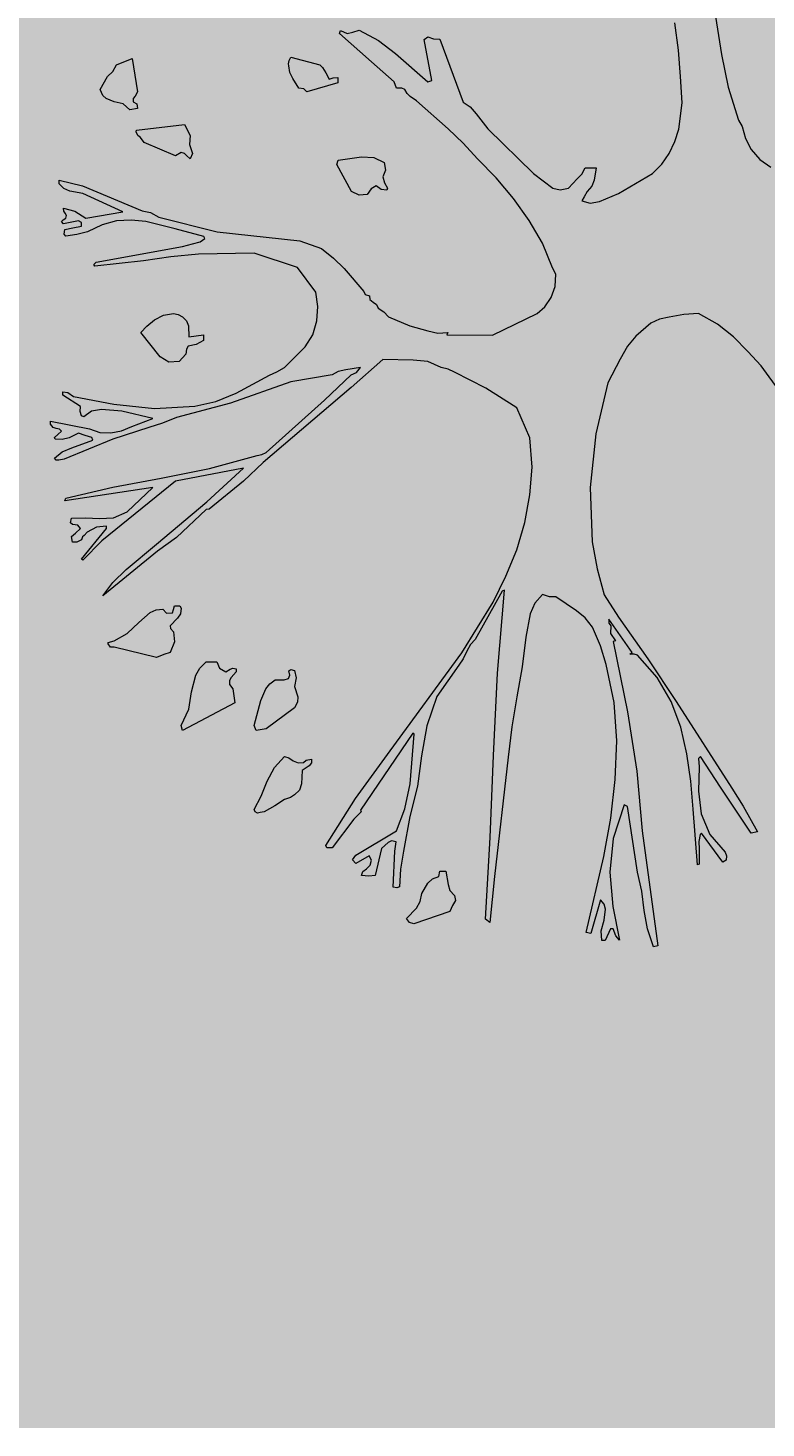
# Model space of a CAD drawing. Units: inches. Extents: x 84 to 1044, y -280 to 906.
# Tile 87 of 105: x 870 to 883, y 400 to 426. Entities that reach past the tile are written whole.
import ezdxf

# ---------------------------------------------------------------- set-up
doc = ezdxf.new("R2010")
doc.units = ezdxf.units.IN
doc.layers.add('A-ANNO-DIMS', color=2, linetype='Continuous', lineweight=18)
doc.layers.add('L-PLNT', color=114, linetype='Continuous', lineweight=15)
doc.layers.add('L-PLNT-PATT', color=9, linetype='Continuous', lineweight=9, true_color=0xafd9aa)
doc.styles.get("Standard").update_dxf_attribs({"font": 'arial.ttf'})
doc.dimstyles.get("Standard").update_dxf_attribs({"dimtxt": 0.18, "dimasz": 0.18, "dimexe": 0.18, "dimexo": 0.0625, "dimgap": 0.09, "dimtad": 0, "dimtih": 1, "dimtoh": 1, "dimdec": 4, "dimzin": 0, "dimdsep": 46, "dimtxsty": 'Standard', "dimcen": 0.09, "dimadec": 0, "dimazin": 0, "dimtfac": 1, "dimtdec": 4, "dimtofl": 0, "dimtmove": 0, "dimatfit": 3, "dimfxl": 1, "dimtolj": 1, "dimtzin": 0, "dimarcsym": 0})

# ---------------------------------------------------------------- blocks, each defined once
blk = doc.blocks.new('A$C37E508DF')
for p, q in [((0.7911, 1.1436), (0.8027, 1.0677)), ((0.3456, 1.093), (0.3469, 1.0964)), ((0.3842, 1.0591), (0.3456, 1.093)), ((0.3469, 1.0964), (0.355, 1.093)), ((0.355, 1.093), (0.3619, 1.0943)), ((0.3619, 1.0943), (0.3692, 1.0968)), ((0.3692, 1.0968), (0.3923, 1.0844)), ((0.7512, 1.0728), (0.7469, 1.1054)), ((0.3923, 1.0844), (0.4129, 1.069)), ((0.4472, 1.0857), (0.4515, 1.0887)), ((0.4562, 1.0364), (0.4472, 1.0857)), ((0.4515, 1.0887), (0.4584, 1.0865)), ((0.4584, 1.0865), (0.4657, 1.0861)), ((0.4657, 1.0861), (0.4939, 1.0107)), ((0.7538, 1.0415), (0.7512, 1.0728)), ((0.0789, 1.0552), (0.0978, 1.063)), ((0.0978, 1.063), (0.1042, 1.0231)), ((0.2847, 1.0565), (0.2856, 1.0604)), ((0.2851, 1.054), (0.2847, 1.0565)), ((0.2856, 1.0604), (0.2877, 1.0647)), ((0.2877, 1.0647), (0.3224, 1.0552)), ((0.4112, 1.0351), (0.3842, 1.0591)), ((0.4129, 1.069), (0.4515, 1.0351)), ((0.8027, 1.0677), (0.8108, 1.0287)), ((0.0596, 1.0257), (0.0682, 1.0415)), ((0.0682, 1.0415), (0.0746, 1.0475)), ((0.0746, 1.0475), (0.0789, 1.0552)), ((0.2864, 1.0463), (0.2851, 1.054)), ((0.2899, 1.039), (0.2864, 1.0463)), ((0.2972, 1.0274), (0.2899, 1.039)), ((0.3224, 1.0552), (0.3255, 1.0522)), ((0.3255, 1.0522), (0.3293, 1.0458)), ((0.3293, 1.0458), (0.3336, 1.0381)), ((0.3336, 1.0381), (0.3383, 1.0398)), ((0.3383, 1.0398), (0.3439, 1.0402)), ((0.3439, 1.0402), (0.3439, 1.0338)), ((0.7559, 1.0098), (0.7538, 1.0415)), ((0.0626, 1.0188), (0.0596, 1.0257)), ((0.1042, 1.0231), (0.1012, 1.018)), ((0.3032, 1.0265), (0.2972, 1.0274)), ((0.3066, 1.0231), (0.3032, 1.0265)), ((0.3439, 1.0338), (0.3066, 1.0231)), ((0.4138, 1.0274), (0.4112, 1.0351)), ((0.4202, 1.0274), (0.4138, 1.0274)), ((0.4241, 1.0257), (0.4202, 1.0274)), ((0.4267, 1.0209), (0.4241, 1.0257)), ((0.4515, 1.0351), (0.4562, 1.0364)), ((0.8108, 1.0287), (0.8233, 0.9892)), ((0.0665, 1.0149), (0.0626, 1.0188)), ((0.0763, 1.0111), (0.0665, 1.0149)), ((0.087, 1.0085), (0.0763, 1.0111)), ((0.0948, 1.0016), (0.087, 1.0085)), ((0.1012, 1.018), (0.099, 1.0149)), ((0.099, 1.0149), (0.099, 1.0111)), ((0.099, 1.0111), (0.1033, 1.0085)), ((0.1033, 1.0085), (0.1042, 1.0029)), ((0.4305, 1.0175), (0.4267, 1.0209)), ((0.4378, 1.0124), (0.4305, 1.0175)), ((0.476, 0.9789), (0.4378, 1.0124)), ((0.4939, 1.0107), (0.5021, 1.0051)), ((0.5021, 1.0051), (0.5094, 0.9969)), ((0.7516, 0.9785), (0.7559, 1.0098)), ((0.1042, 1.0029), (0.0948, 1.0016)), ((0.5094, 0.9969), (0.5231, 0.9789)), ((0.8233, 0.9892), (0.8275, 0.9815)), ((0.1025, 0.9751), (0.1029, 0.9772)), ((0.1046, 0.9708), (0.1025, 0.9751)), ((0.1029, 0.9772), (0.1604, 0.9841)), ((0.1604, 0.9841), (0.1672, 0.9708)), ((0.4939, 0.9618), (0.476, 0.9789)), ((0.5231, 0.9789), (0.578, 0.9253)), ((0.7469, 0.9635), (0.7516, 0.9785)), ((0.8275, 0.9815), (0.8314, 0.9673)), ((0.1076, 0.9682), (0.1046, 0.9708)), ((0.1119, 0.9626), (0.1076, 0.9682)), ((0.1496, 0.9463), (0.1119, 0.9626)), ((0.1672, 0.9708), (0.1664, 0.9601)), ((0.1664, 0.9601), (0.1698, 0.9493)), ((0.5111, 0.9429), (0.4939, 0.9618)), ((0.7401, 0.9493), (0.7469, 0.9635)), ((0.8314, 0.9673), (0.8383, 0.954)), ((0.1565, 0.9506), (0.1496, 0.9463)), ((0.1604, 0.9493), (0.1565, 0.9506)), ((0.1629, 0.9468), (0.1604, 0.9493)), ((0.1672, 0.9429), (0.1629, 0.9468)), ((0.1698, 0.9493), (0.1672, 0.9429)), ((0.3426, 0.936), (0.3443, 0.9412)), ((0.3443, 0.9412), (0.3722, 0.9451)), ((0.3722, 0.9451), (0.3868, 0.9446)), ((0.3868, 0.9446), (0.3992, 0.9386)), ((0.3992, 0.9386), (0.4009, 0.9292)), ((0.5334, 0.9202), (0.5111, 0.9429)), ((0.7315, 0.9365), (0.7401, 0.9493)), ((0.8383, 0.954), (0.8486, 0.942)), ((0.8486, 0.942), (0.8619, 0.933)), ((0.3602, 0.9039), (0.3426, 0.936)), ((0.4009, 0.9292), (0.3975, 0.9215)), ((0.3975, 0.9215), (0.3996, 0.9142)), ((0.578, 0.9253), (0.6011, 0.9077)), ((0.6303, 0.9189), (0.6359, 0.9245)), ((0.6359, 0.9245), (0.6397, 0.9322)), ((0.6397, 0.9322), (0.653, 0.9322)), ((0.653, 0.9322), (0.6505, 0.9172)), ((0.6796, 0.9013), (0.7203, 0.9253)), ((0.7203, 0.9253), (0.7315, 0.9365)), ((0.0103, 0.9129), (0.0103, 0.9172)), ((0.0103, 0.9172), (0.0382, 0.9107)), ((0.0159, 0.9073), (0.0103, 0.9129)), ((0.0232, 0.9043), (0.0159, 0.9073)), ((0.0382, 0.9107), (0.1098, 0.8807)), ((0.3838, 0.9069), (0.379, 0.9)), ((0.3898, 0.9107), (0.3838, 0.9069)), ((0.3958, 0.906), (0.3898, 0.9107)), ((0.4026, 0.9052), (0.3958, 0.906)), ((0.3996, 0.9142), (0.4031, 0.9077)), ((0.4031, 0.9077), (0.4026, 0.9052)), ((0.554, 0.8953), (0.5334, 0.9202)), ((0.6011, 0.9077), (0.6097, 0.9056)), ((0.6097, 0.9056), (0.6196, 0.9077)), ((0.6196, 0.9077), (0.6303, 0.9189)), ((0.6479, 0.9103), (0.6423, 0.9039)), ((0.6505, 0.9172), (0.6479, 0.9103)), ((0.0386, 0.9013), (0.0232, 0.9043)), ((0.0866, 0.8794), (0.0386, 0.9013)), ((0.3692, 0.8992), (0.3602, 0.9039)), ((0.379, 0.9), (0.3692, 0.8992)), ((0.5728, 0.8691), (0.554, 0.8953)), ((0.6384, 0.8974), (0.6359, 0.8927)), ((0.6359, 0.8927), (0.6457, 0.8897)), ((0.6423, 0.9039), (0.6384, 0.8974)), ((0.6457, 0.8897), (0.6569, 0.8919)), ((0.6569, 0.8919), (0.6796, 0.9013)), ((0.015, 0.87), (0.0184, 0.8717)), ((0.0159, 0.8803), (0.0154, 0.8837)), ((0.0154, 0.8837), (0.0292, 0.8803)), ((0.0176, 0.8777), (0.0159, 0.8803)), ((0.0193, 0.8752), (0.0176, 0.8777)), ((0.0184, 0.8717), (0.0193, 0.8752)), ((0.0292, 0.8803), (0.0424, 0.8717)), ((0.0424, 0.8717), (0.0866, 0.8794)), ((0.1098, 0.8807), (0.1196, 0.8786)), ((0.1196, 0.8786), (0.1295, 0.873)), ((0.1295, 0.873), (0.1994, 0.8554)), ((0.0133, 0.8679), (0.015, 0.87)), ((0.0154, 0.8649), (0.0133, 0.8679)), ((0.0334, 0.8687), (0.0154, 0.8649)), ((0.0163, 0.8529), (0.0171, 0.8584)), ((0.0171, 0.8584), (0.0266, 0.8602)), ((0.0266, 0.8602), (0.0369, 0.8623)), ((0.0442, 0.8554), (0.0317, 0.8524)), ((0.0369, 0.8666), (0.0334, 0.8687)), ((0.0369, 0.8623), (0.0369, 0.8666)), ((0.0617, 0.864), (0.0442, 0.8554)), ((0.0789, 0.8687), (0.0617, 0.864)), ((0.0965, 0.8696), (0.0789, 0.8687)), ((0.1141, 0.8679), (0.0965, 0.8696)), ((0.1492, 0.8593), (0.1141, 0.8679)), ((0.1835, 0.8499), (0.1492, 0.8593)), ((0.1994, 0.8554), (0.2984, 0.8447)), ((0.5887, 0.8421), (0.5728, 0.8691)), ((0.0184, 0.8503), (0.0163, 0.8529)), ((0.0317, 0.8524), (0.0184, 0.8503)), ((0.0545, 0.8194), (0.1578, 0.8378)), ((0.1578, 0.8378), (0.1698, 0.8413)), ((0.1698, 0.8413), (0.1792, 0.8434)), ((0.1792, 0.8434), (0.1848, 0.8477)), ((0.1848, 0.8477), (0.1835, 0.8499)), ((0.2984, 0.8447), (0.3242, 0.8357)), ((0.6007, 0.8125), (0.5887, 0.8421)), ((0.1441, 0.8258), (0.1111, 0.8207)), ((0.1771, 0.8288), (0.1441, 0.8258)), ((0.2436, 0.8301), (0.1771, 0.8288)), ((0.2954, 0.813), (0.2436, 0.8301)), ((0.3242, 0.8357), (0.3387, 0.8241)), ((0.3387, 0.8241), (0.3512, 0.8117)), ((0.0519, 0.8164), (0.0545, 0.8194)), ((0.0532, 0.8143), (0.0519, 0.8164)), ((0.1111, 0.8207), (0.0532, 0.8143)), ((0.3173, 0.7834), (0.2954, 0.813)), ((0.3512, 0.8117), (0.3748, 0.7842)), ((0.6046, 0.8048), (0.6007, 0.8125)), ((0.6037, 0.7903), (0.6046, 0.8048)), ((0.599, 0.777), (0.6037, 0.7903)), ((0.3199, 0.7662), (0.3173, 0.7834)), ((0.3748, 0.7842), (0.3765, 0.7804)), ((0.3765, 0.7804), (0.3816, 0.7791)), ((0.3816, 0.7791), (0.382, 0.7744)), ((0.382, 0.7744), (0.3859, 0.7714)), ((0.3859, 0.7714), (0.3902, 0.7684)), ((0.5913, 0.7658), (0.599, 0.777)), ((0.1244, 0.7504), (0.1351, 0.7559)), ((0.1351, 0.7559), (0.1471, 0.7577)), ((0.1471, 0.7577), (0.1527, 0.7568)), ((0.1527, 0.7568), (0.1578, 0.7538)), ((0.1578, 0.7538), (0.1629, 0.7491)), ((0.3186, 0.7491), (0.3199, 0.7662)), ((0.3902, 0.7684), (0.3919, 0.7641)), ((0.3919, 0.7641), (0.3988, 0.7598)), ((0.3988, 0.7598), (0.4043, 0.7538)), ((0.4043, 0.7538), (0.4301, 0.7431)), ((0.5287, 0.7319), (0.5823, 0.7577)), ((0.5823, 0.7577), (0.5913, 0.7658)), ((0.7577, 0.7568), (0.7401, 0.7534)), ((0.7752, 0.7577), (0.7577, 0.7568)), ((0.798, 0.7452), (0.7752, 0.7577)), ((0.1081, 0.7349), (0.1153, 0.7427)), ((0.1153, 0.7427), (0.1244, 0.7504)), ((0.1629, 0.7491), (0.1651, 0.7431)), ((0.1651, 0.7431), (0.1655, 0.7298)), ((0.3139, 0.7324), (0.3186, 0.7491)), ((0.4301, 0.7431), (0.4515, 0.7371)), ((0.4515, 0.7371), (0.4635, 0.7341)), ((0.7182, 0.7461), (0.7002, 0.7307)), ((0.7285, 0.7512), (0.7182, 0.7461)), ((0.7401, 0.7534), (0.7285, 0.7512)), ((0.8173, 0.7298), (0.798, 0.7452)), ((0.1312, 0.7058), (0.1081, 0.7349)), ((0.1741, 0.7208), (0.1646, 0.7186)), ((0.1655, 0.7298), (0.1831, 0.7324)), ((0.1831, 0.7255), (0.1741, 0.7208)), ((0.1831, 0.7324), (0.1831, 0.7255)), ((0.3049, 0.7178), (0.3139, 0.7324)), ((0.4635, 0.7341), (0.4755, 0.7349)), ((0.4755, 0.7349), (0.4742, 0.7324)), ((0.4742, 0.7324), (0.5287, 0.7319)), ((0.7002, 0.7307), (0.6903, 0.7186)), ((0.8344, 0.7122), (0.8173, 0.7298)), ((0.1415, 0.6994), (0.1312, 0.7058)), ((0.1621, 0.7092), (0.1539, 0.7002)), ((0.1629, 0.7152), (0.1621, 0.7092)), ((0.1646, 0.7186), (0.1629, 0.7152)), ((0.28, 0.6933), (0.3049, 0.7178)), ((0.6903, 0.7186), (0.6818, 0.7032)), ((0.8503, 0.6951), (0.8344, 0.7122)), ((0.1539, 0.7002), (0.1415, 0.6994)), ((0.262, 0.6839), (0.271, 0.6882)), ((0.271, 0.6882), (0.28, 0.6933)), ((0.3443, 0.6886), (0.337, 0.6843)), ((0.3533, 0.6903), (0.3443, 0.6886)), ((0.3709, 0.6933), (0.3533, 0.6903)), ((0.3975, 0.7028), (0.3598, 0.6693)), ((0.3598, 0.6843), (0.3662, 0.6873)), ((0.3662, 0.6873), (0.3709, 0.6933)), ((0.4339, 0.7019), (0.3975, 0.7028)), ((0.4515, 0.7002), (0.4339, 0.7019)), ((0.4674, 0.6933), (0.4515, 0.7002)), ((0.476, 0.6912), (0.4674, 0.6933)), ((0.4832, 0.6878), (0.476, 0.6912)), ((0.521, 0.6685), (0.4832, 0.6878)), ((0.6818, 0.7032), (0.6667, 0.6749)), ((0.8739, 0.6629), (0.8503, 0.6951)), ((0.2877, 0.6762), (0.2152, 0.6505)), ((0.2221, 0.6625), (0.262, 0.6839)), ((0.337, 0.6843), (0.2877, 0.6762)), ((0.328, 0.6543), (0.3598, 0.6843)), ((0.6667, 0.6749), (0.6526, 0.614)), ((0.0146, 0.6599), (0.0146, 0.6642)), ((0.0146, 0.6642), (0.0206, 0.6633)), ((0.036, 0.6466), (0.0146, 0.6599)), ((0.0206, 0.6633), (0.0274, 0.6586)), ((0.0274, 0.6586), (0.0759, 0.6492)), ((0.1977, 0.6526), (0.2221, 0.6625)), ((0.3598, 0.6693), (0.2543, 0.5797)), ((0.2581, 0.5913), (0.328, 0.6543)), ((0.5578, 0.6449), (0.521, 0.6685)), ((0.0356, 0.6406), (0.036, 0.6466)), ((0.0369, 0.6355), (0.0356, 0.6406)), ((0.0489, 0.641), (0.0399, 0.6342)), ((0.0609, 0.6428), (0.0489, 0.641)), ((0.0853, 0.641), (0.0609, 0.6428)), ((0.0759, 0.6492), (0.1244, 0.644)), ((0.1226, 0.632), (0.0853, 0.641)), ((0.1244, 0.644), (0.1728, 0.647)), ((0.2152, 0.6505), (0.1509, 0.6333)), ((0.1728, 0.647), (0.1977, 0.6526)), ((0.5737, 0.6089), (0.5578, 0.6449)), ((0, 0.629), (0.0467, 0.62)), ((0, 0.6252), (0, 0.629)), ((0.003, 0.6213), (0, 0.6252)), ((0.0069, 0.6204), (0.003, 0.6213)), ((0.0107, 0.6196), (0.0069, 0.6204)), ((0.0399, 0.6342), (0.0369, 0.6355)), ((0.0467, 0.62), (0.0592, 0.6153)), ((0.1175, 0.6213), (0.0746, 0.6076)), ((0.0849, 0.6175), (0.0973, 0.6226)), ((0.0973, 0.6226), (0.1226, 0.632)), ((0.1342, 0.6265), (0.1175, 0.6213)), ((0.1509, 0.6333), (0.1342, 0.6265)), ((0.0047, 0.6093), (0.0086, 0.6132)), ((0.0056, 0.6076), (0.0047, 0.6093)), ((0.0141, 0.6072), (0.0056, 0.6076)), ((0.0086, 0.6132), (0.0133, 0.617)), ((0.0133, 0.617), (0.0107, 0.6196)), ((0.0223, 0.6089), (0.0141, 0.6072)), ((0.0746, 0.6076), (0.0163, 0.5836)), ((0.0334, 0.6145), (0.0223, 0.6089)), ((0.0257, 0.5969), (0.0506, 0.6063)), ((0.0416, 0.6119), (0.0334, 0.6145)), ((0.0493, 0.6093), (0.0416, 0.6119)), ((0.0506, 0.6063), (0.0493, 0.6093)), ((0.0592, 0.6153), (0.072, 0.6149)), ((0.072, 0.6149), (0.0849, 0.6175)), ((0.5763, 0.5741), (0.5737, 0.6089)), ((0.6526, 0.614), (0.6457, 0.5497)), ((0.0047, 0.5849), (0.0141, 0.5921)), ((0.0141, 0.5921), (0.0257, 0.5969)), ((0.1904, 0.5724), (0.2474, 0.5879)), ((0.2474, 0.5879), (0.253, 0.5892)), ((0.253, 0.5892), (0.2581, 0.5913)), ((0.0069, 0.5823), (0.0047, 0.5849)), ((0.0099, 0.5823), (0.0069, 0.5823)), ((0.0163, 0.5836), (0.0099, 0.5823)), ((0.1325, 0.5608), (0.1904, 0.5724)), ((0.2311, 0.5729), (0.1496, 0.557)), ((0.1869, 0.5325), (0.2311, 0.5729)), ((0.2543, 0.5797), (0.2311, 0.557)), ((0.5737, 0.5407), (0.5763, 0.5741)), ((0.1496, 0.557), (0.0613, 0.4858)), ((0.0746, 0.5501), (0.1325, 0.5608)), ((0.2311, 0.557), (0.1899, 0.5235)), ((0.1226, 0.5497), (0.0171, 0.5338)), ((0.0171, 0.5338), (0.0184, 0.5368)), ((0.0184, 0.5368), (0.0746, 0.5501)), ((0.0917, 0.5205), (0.1226, 0.5497)), ((0.5677, 0.5077), (0.5737, 0.5407)), ((0.6457, 0.5497), (0.6483, 0.4845)), ((0.0755, 0.5133), (0.0917, 0.5205)), ((0.1269, 0.482), (0.1869, 0.5325)), ((0.1861, 0.5231), (0.1509, 0.4897)), ((0.1899, 0.5235), (0.1861, 0.5231)), ((0.024, 0.5072), (0.0253, 0.5128)), ((0.0262, 0.5055), (0.024, 0.5072)), ((0.0253, 0.5128), (0.042, 0.5133)), ((0.0326, 0.5047), (0.0262, 0.5055)), ((0.036, 0.5004), (0.0326, 0.5047)), ((0.042, 0.5133), (0.0587, 0.5124)), ((0.0669, 0.5034), (0.0549, 0.5021)), ((0.0587, 0.5124), (0.0755, 0.5133)), ((0.0669, 0.5004), (0.0669, 0.5034)), ((0.5578, 0.4751), (0.5677, 0.5077)), ((0.0253, 0.491), (0.03, 0.4948)), ((0.0262, 0.4841), (0.0253, 0.491)), ((0.03, 0.4948), (0.036, 0.5004)), ((0.0369, 0.4871), (0.0317, 0.4841)), ((0.0369, 0.4639), (0.0669, 0.5004)), ((0.0382, 0.4905), (0.0369, 0.4871)), ((0.0403, 0.4922), (0.0382, 0.4905)), ((0.0613, 0.4858), (0.0386, 0.4627)), ((0.0437, 0.4961), (0.0403, 0.4922)), ((0.0549, 0.5021), (0.0437, 0.4961)), ((0.1509, 0.4897), (0.1282, 0.4734)), ((0.0317, 0.4841), (0.0262, 0.4841)), ((0.1282, 0.4734), (0.0626, 0.4198)), ((0.0905, 0.4515), (0.1269, 0.482)), ((0.545, 0.4434), (0.5578, 0.4751)), ((0.6483, 0.4845), (0.6539, 0.4524)), ((0.0386, 0.4627), (0.0369, 0.4639)), ((0.6539, 0.4524), (0.6625, 0.4211)), ((0.0626, 0.4198), (0.0746, 0.4361)), ((0.0746, 0.4361), (0.0905, 0.4515)), ((0.5295, 0.4125), (0.545, 0.4434)), ((0.5403, 0.4254), (0.5081, 0.3679)), ((0.5347, 0.3276), (0.5433, 0.4266)), ((0.5433, 0.4266), (0.5403, 0.4254)), ((0.5887, 0.4215), (0.5797, 0.4112)), ((0.5969, 0.4189), (0.5887, 0.4215)), ((0.6046, 0.4189), (0.5969, 0.4189)), ((0.6295, 0.4022), (0.6046, 0.4189)), ((0.6625, 0.4211), (0.6796, 0.3945)), ((0.1192, 0.4001), (0.1265, 0.4031)), ((0.1265, 0.4031), (0.1346, 0.4039)), ((0.1346, 0.4039), (0.1389, 0.3992)), ((0.1458, 0.3996), (0.1471, 0.4035)), ((0.1471, 0.4035), (0.1484, 0.4082)), ((0.1484, 0.4082), (0.1548, 0.4082)), ((0.1548, 0.4082), (0.1565, 0.4052)), ((0.1565, 0.4052), (0.1556, 0.3983)), ((0.4922, 0.3516), (0.5295, 0.4125)), ((0.5797, 0.4112), (0.5741, 0.3983)), ((0.6397, 0.3936), (0.6295, 0.4022)), ((0.0917, 0.3748), (0.1055, 0.388)), ((0.1055, 0.388), (0.1192, 0.4001)), ((0.1389, 0.3992), (0.1458, 0.3996)), ((0.1518, 0.3932), (0.1432, 0.3842)), ((0.1556, 0.3983), (0.1518, 0.3932)), ((0.5741, 0.3983), (0.5686, 0.3705)), ((0.6487, 0.3825), (0.6397, 0.3936)), ((0.6959, 0.352), (0.668, 0.3919)), ((0.668, 0.3919), (0.668, 0.3872)), ((0.668, 0.3872), (0.6706, 0.3842)), ((0.6796, 0.3945), (0.7148, 0.3447)), ((0.0763, 0.3662), (0.0917, 0.3748)), ((0.1432, 0.3842), (0.1436, 0.3808)), ((0.1436, 0.3808), (0.1471, 0.3769)), ((0.1471, 0.3769), (0.1484, 0.3649)), ((0.5686, 0.3705), (0.5643, 0.3349)), ((0.6582, 0.3602), (0.6487, 0.3825)), ((0.6706, 0.3842), (0.6702, 0.3748)), ((0.6702, 0.3748), (0.6762, 0.3662)), ((0.069, 0.364), (0.0763, 0.3662)), ((0.069, 0.3627), (0.069, 0.364)), ((0.0716, 0.3585), (0.069, 0.3627)), ((0.0763, 0.3585), (0.0716, 0.3585)), ((0.1269, 0.3464), (0.0763, 0.3585)), ((0.1432, 0.352), (0.1355, 0.3499)), ((0.1484, 0.3649), (0.1432, 0.352)), ((0.4982, 0.3537), (0.4939, 0.3447)), ((0.5025, 0.3619), (0.4982, 0.3537)), ((0.5081, 0.3679), (0.5025, 0.3619)), ((0.665, 0.3379), (0.6582, 0.3602)), ((0.6762, 0.3662), (0.6732, 0.3653)), ((0.6732, 0.3653), (0.6903, 0.2813)), ((0.6933, 0.3503), (0.6959, 0.352)), ((0.1355, 0.3499), (0.1269, 0.3464)), ((0.1788, 0.3336), (0.1861, 0.3409)), ((0.1861, 0.3409), (0.199, 0.3409)), ((0.199, 0.3409), (0.2024, 0.3336)), ((0.4065, 0.2345), (0.4922, 0.3516)), ((0.4884, 0.337), (0.4622, 0.2997)), ((0.4939, 0.3447), (0.4884, 0.337)), ((0.6745, 0.2924), (0.665, 0.3379)), ((0.6985, 0.3503), (0.6933, 0.3503)), ((0.7023, 0.349), (0.6985, 0.3503)), ((0.7259, 0.3224), (0.7023, 0.349)), ((0.7148, 0.3447), (0.7487, 0.2937)), ((0.1689, 0.3053), (0.1737, 0.325)), ((0.1737, 0.325), (0.1788, 0.3336)), ((0.2024, 0.3336), (0.2097, 0.3289)), ((0.2097, 0.3289), (0.2148, 0.3323)), ((0.2161, 0.3224), (0.214, 0.3186)), ((0.214, 0.3186), (0.214, 0.3139)), ((0.2148, 0.3323), (0.2182, 0.3336)), ((0.2221, 0.3289), (0.2161, 0.3224)), ((0.2182, 0.3336), (0.2221, 0.3327)), ((0.2221, 0.3327), (0.2221, 0.3289)), ((0.2624, 0.3147), (0.2689, 0.3194)), ((0.2689, 0.3194), (0.2796, 0.3194)), ((0.2796, 0.3194), (0.2847, 0.3211)), ((0.2847, 0.3211), (0.2864, 0.325)), ((0.2851, 0.3302), (0.2877, 0.3319)), ((0.2864, 0.325), (0.2851, 0.3302)), ((0.2877, 0.3319), (0.292, 0.3306)), ((0.292, 0.3306), (0.2941, 0.322)), ((0.2941, 0.322), (0.292, 0.3117)), ((0.53, 0.229), (0.5347, 0.3276)), ((0.5643, 0.3349), (0.5578, 0.2993)), ((0.7427, 0.2937), (0.7259, 0.3224)), ((0.1655, 0.2843), (0.1689, 0.3053)), ((0.214, 0.3139), (0.2182, 0.3087)), ((0.2182, 0.3087), (0.2204, 0.292)), ((0.2517, 0.2946), (0.2577, 0.3087)), ((0.2577, 0.3087), (0.2624, 0.3147)), ((0.292, 0.3117), (0.2959, 0.2993)), ((0.2204, 0.292), (0.1578, 0.259)), ((0.2436, 0.265), (0.2517, 0.2946)), ((0.292, 0.286), (0.2581, 0.2607)), ((0.2954, 0.2928), (0.292, 0.286)), ((0.2959, 0.2993), (0.2954, 0.2928)), ((0.4622, 0.2997), (0.4502, 0.2645)), ((0.5578, 0.2993), (0.5518, 0.2633)), ((0.6775, 0.2465), (0.6745, 0.2924)), ((0.7542, 0.2628), (0.7427, 0.2937)), ((0.7487, 0.2937), (0.8151, 0.1899)), ((0.1565, 0.265), (0.1655, 0.2843)), ((0.6903, 0.2813), (0.7015, 0.2101)), ((0.1578, 0.259), (0.1565, 0.265)), ((0.2461, 0.259), (0.2436, 0.265)), ((0.2581, 0.2607), (0.2461, 0.259)), ((0.4335, 0.2556), (0.3709, 0.1634)), ((0.4305, 0.1951), (0.4352, 0.2543)), ((0.4352, 0.2543), (0.4335, 0.2556)), ((0.4502, 0.2645), (0.4438, 0.2285)), ((0.5518, 0.2633), (0.5475, 0.2268)), ((0.7615, 0.2311), (0.7542, 0.2628)), ((0.3649, 0.1775), (0.4065, 0.2345)), ((0.6758, 0.2002), (0.6775, 0.2465)), ((0.268, 0.2148), (0.28, 0.2277)), ((0.28, 0.2277), (0.2851, 0.226)), ((0.2851, 0.226), (0.2903, 0.2225)), ((0.2903, 0.2225), (0.2963, 0.22)), ((0.2963, 0.22), (0.3027, 0.2204)), ((0.3027, 0.2204), (0.3061, 0.2234)), ((0.3061, 0.2234), (0.3122, 0.2247)), ((0.3122, 0.22), (0.3096, 0.2165)), ((0.3122, 0.2247), (0.3122, 0.22)), ((0.4438, 0.2285), (0.4391, 0.1921)), ((0.5261, 0.1308), (0.53, 0.229)), ((0.5475, 0.2268), (0.5313, 0.084)), ((0.7662, 0.1981), (0.7615, 0.2311)), ((0.7778, 0.2277), (0.7752, 0.2255)), ((0.7752, 0.2255), (0.7761, 0.2152)), ((0.8018, 0.1912), (0.7778, 0.2277)), ((0.2594, 0.1981), (0.268, 0.2148)), ((0.301, 0.211), (0.3002, 0.1951)), ((0.3096, 0.2165), (0.301, 0.211)), ((0.7015, 0.2101), (0.7079, 0.1389)), ((0.7761, 0.2152), (0.7752, 0.1861)), ((0.2521, 0.1805), (0.2594, 0.1981)), ((0.298, 0.1874), (0.292, 0.1818)), ((0.3002, 0.1951), (0.298, 0.1874)), ((0.4241, 0.1651), (0.4305, 0.1951)), ((0.4391, 0.1921), (0.4301, 0.1561)), ((0.6706, 0.1539), (0.6758, 0.2002)), ((0.7688, 0.1646), (0.7662, 0.1981)), ((0.7752, 0.1861), (0.7787, 0.1591)), ((0.8383, 0.1359), (0.8018, 0.1912)), ((0.8151, 0.1899), (0.8288, 0.1685)), ((0.2436, 0.1642), (0.2521, 0.1805)), ((0.2684, 0.1689), (0.2556, 0.1616)), ((0.28, 0.1762), (0.2684, 0.1689)), ((0.2873, 0.1788), (0.28, 0.1762)), ((0.292, 0.1818), (0.2873, 0.1788)), ((0.3293, 0.1213), (0.3649, 0.1775)), ((0.6865, 0.1698), (0.6732, 0.1295)), ((0.6903, 0.1681), (0.6865, 0.1698)), ((0.7023, 0.0892), (0.6903, 0.1681)), ((0.8288, 0.1685), (0.846, 0.1376)), ((0.2448, 0.1616), (0.2436, 0.1642)), ((0.2478, 0.1599), (0.2448, 0.1616)), ((0.2508, 0.1608), (0.2478, 0.1599)), ((0.2556, 0.1616), (0.2508, 0.1608)), ((0.3628, 0.1526), (0.337, 0.1183)), ((0.3692, 0.1591), (0.3628, 0.1526)), ((0.3718, 0.1616), (0.3692, 0.1591)), ((0.3709, 0.1634), (0.3718, 0.1616)), ((0.4138, 0.1389), (0.4241, 0.1651)), ((0.4301, 0.1561), (0.4224, 0.1145)), ((0.662, 0.108), (0.6706, 0.1539)), ((0.774, 0.0982), (0.7688, 0.1646)), ((0.7787, 0.1591), (0.789, 0.1346)), ((0.3653, 0.1098), (0.4138, 0.1389)), ((0.7079, 0.1389), (0.7268, 0.0013)), ((0.7774, 0.1346), (0.7757, 0.1261)), ((0.7791, 0.1359), (0.7774, 0.1346)), ((0.8044, 0.1012), (0.7791, 0.1359)), ((0.789, 0.1346), (0.8074, 0.1132)), ((0.846, 0.1376), (0.8383, 0.1359)), ((0.3306, 0.1183), (0.3293, 0.1213)), ((0.337, 0.1183), (0.3306, 0.1183)), ((0.3962, 0.1175), (0.3885, 0.0853)), ((0.4039, 0.1248), (0.3962, 0.1175)), ((0.4082, 0.1269), (0.4039, 0.1248)), ((0.4134, 0.1256), (0.4082, 0.1269)), ((0.4121, 0.1145), (0.4134, 0.1256)), ((0.5205, 0.033), (0.5261, 0.1308)), ((0.6732, 0.1295), (0.6693, 0.0892)), ((0.7757, 0.1261), (0.7761, 0.117)), ((0.3615, 0.1042), (0.3653, 0.1098)), ((0.3653, 0.0999), (0.3615, 0.1042)), ((0.3812, 0.1089), (0.3653, 0.0999)), ((0.3842, 0.1037), (0.3812, 0.1089)), ((0.3825, 0.0978), (0.3842, 0.1037)), ((0.4099, 0.0716), (0.4121, 0.1145)), ((0.4224, 0.1145), (0.4189, 0.093)), ((0.641, 0.0172), (0.662, 0.108)), ((0.7761, 0.117), (0.7761, 0.099)), ((0.8083, 0.1037), (0.8044, 0.1012)), ((0.8074, 0.1132), (0.8087, 0.1089)), ((0.8087, 0.1089), (0.8083, 0.1037)), ((0.3722, 0.0853), (0.3739, 0.09)), ((0.3808, 0.0845), (0.3722, 0.0853)), ((0.3739, 0.09), (0.3782, 0.0935)), ((0.3782, 0.0935), (0.3825, 0.0978)), ((0.3885, 0.0853), (0.3808, 0.0845)), ((0.4189, 0.093), (0.4176, 0.072)), ((0.4571, 0.0815), (0.4648, 0.084)), ((0.4648, 0.084), (0.4657, 0.0905)), ((0.4657, 0.0905), (0.473, 0.0905)), ((0.473, 0.0905), (0.476, 0.0746)), ((0.5313, 0.084), (0.5257, 0.0291)), ((0.6693, 0.0892), (0.6728, 0.0484)), ((0.7075, 0.0665), (0.7023, 0.0892)), ((0.7761, 0.099), (0.774, 0.0982)), ((0.4142, 0.0707), (0.4099, 0.0716)), ((0.4176, 0.072), (0.4142, 0.0707)), ((0.4442, 0.0639), (0.4515, 0.0763)), ((0.4515, 0.0763), (0.4571, 0.0815)), ((0.476, 0.0746), (0.4777, 0.0673)), ((0.4777, 0.0673), (0.4832, 0.0613)), ((0.4378, 0.0463), (0.4425, 0.0544)), ((0.4425, 0.0544), (0.4442, 0.0639)), ((0.4845, 0.0553), (0.4811, 0.0493)), ((0.4832, 0.0613), (0.4845, 0.0553)), ((0.6582, 0.0562), (0.6466, 0.0159)), ((0.6625, 0.051), (0.6582, 0.0562)), ((0.6642, 0.045), (0.6625, 0.051)), ((0.7105, 0.0437), (0.7075, 0.0665)), ((0.4258, 0.0339), (0.4378, 0.0463)), ((0.4296, 0.0291), (0.4258, 0.0339)), ((0.4777, 0.0424), (0.4348, 0.0274)), ((0.4811, 0.0493), (0.4777, 0.0424)), ((0.6625, 0.0321), (0.6642, 0.045)), ((0.6728, 0.0484), (0.6809, 0.0082)), ((0.7144, 0.0214), (0.7105, 0.0437)), ((0.4348, 0.0274), (0.4296, 0.0291)), ((0.5257, 0.0291), (0.5205, 0.033)), ((0.6466, 0.0159), (0.641, 0.0172)), ((0.659, 0.0193), (0.6625, 0.0321)), ((0.6595, 0.0077), (0.659, 0.0193)), ((0.6702, 0.0214), (0.6637, 0.0077)), ((0.6732, 0.0214), (0.6702, 0.0214)), ((0.6766, 0.0133), (0.6732, 0.0214)), ((0.7216, 0), (0.7144, 0.0214)), ((0.6637, 0.0077), (0.6595, 0.0077)), ((0.6809, 0.0082), (0.6766, 0.0133)), ((0.7268, 0.0013), (0.7216, 0))]:
    blk.add_line(p, q)
blk = doc.blocks.new('*D62')
at = {"layer": 'A-ANNO-DIMS', "color": 0, "lineweight": -2, "transparency": 16777216}
for p, q in [((203.179, 709.183), (203.179, 905.9)), ((203.359, 905.72), (549.232, 905.72)), ((895.894, 905.72), (550.021, 905.72)), ((896.074, 400.183), (896.074, 905.9))]:
    blk.add_line(p, q, dxfattribs=at)
at = {"layer": 'A-ANNO-DIMS', "color": 0, "transparency": 16777216}
for points in [[(203.359, 905.75), (203.359, 905.69), (203.179, 905.72)], [(895.894, 905.75), (895.894, 905.69), (896.074, 905.72)]]:
    blk.add_solid(points, dxfattribs=at)
at = {"layer": 'Defpoints', "color": 0, "transparency": 16777216}
for p in [(896.074, 905.72), (203.179, 709.12), (896.074, 400.12)]:
    blk.add_point(p, dxfattribs=at)
at = {"layer": 'A-ANNO-DIMS', "color": 0, "transparency": 16777216, "insert": (549.627, 905.72), "char_height": 0.18, "attachment_point": 5}
blk.add_mtext('\\A1;692.9', dxfattribs=at)
blk = doc.blocks.new('*D63')
at = {"layer": 'A-ANNO-DIMS', "color": 0, "lineweight": -2, "transparency": 16777216}
for p, q in [((833.136, 709.12), (1043.768, 709.12)), ((1043.588, 708.94), (1043.588, 400.302)), ((1043.588, 91.3), (1043.588, 399.938)), ((896.136, 91.12), (1043.768, 91.12))]:
    blk.add_line(p, q, dxfattribs=at)
at = {"layer": 'A-ANNO-DIMS', "color": 0, "transparency": 16777216}
for points in [[(1043.558, 708.94), (1043.618, 708.94), (1043.588, 709.12)], [(1043.558, 91.3), (1043.618, 91.3), (1043.588, 91.12)]]:
    blk.add_solid(points, dxfattribs=at)
at = {"layer": 'Defpoints', "color": 0, "transparency": 16777216}
for p in [(833.074, 709.12), (1043.588, 709.12), (896.074, 91.12)]:
    blk.add_point(p, dxfattribs=at)
at = {"layer": 'A-ANNO-DIMS', "color": 0, "transparency": 16777216, "insert": (1043.588, 400.12), "char_height": 0.18, "attachment_point": 5}
blk.add_mtext('\\A1;618', dxfattribs=at)

msp = doc.modelspace()

# ---------------------------------------------------------------- hatches: boundary and pattern name
at = {"layer": 'L-PLNT-PATT', "transparency": 33554597}
h = msp.add_hatch(color=256, dxfattribs=at)
h.dxf.hatch_style = 1
h.paths.add_polyline_path([(896.074, 511.12), (704.074, 511.12), (704.074, 491.62), (704.074, 419.62), (704.074, 400.12), (833.074, 400.12), (896.074, 400.12)])

# ---------------------------------------------------------------- block references
at = {"layer": 'L-PLNT', "xscale": 15.19586232982809, "yscale": 15.19586232982809, "zscale": 15.19586232982809}
msp.add_blockref('A$C37E508DF', (870.466, 408.868), dxfattribs=at)

# ---------------------------------------------------------------- dimensions: what is measured, and where the dimension line sits
at = {"layer": 'A-ANNO-DIMS'}
dim = msp.add_linear_dim(base=(896.074, 905.72), p1=(203.179, 709.12), p2=(896.074, 400.12), dimstyle='Standard', override={"dimdec": 1, "dimlfac": 1, "dimrnd": 0, "dimzin": 0, "dimdsep": 46, "dimlunit": 2}, dxfattribs=at)
dim.commit()
dim.dimension.update_dxf_attribs({"geometry": '*D62', "text_midpoint": (549.627, 905.72)})
dim = msp.add_linear_dim(base=(1043.588, 709.12), p1=(896.074, 91.12), p2=(833.074, 709.12), angle=90, dimstyle='Standard', override={"dimdec": 0, "dimlfac": 1, "dimrnd": 0, "dimzin": 0, "dimdsep": 46, "dimlunit": 2}, dxfattribs=at)
dim.commit()
dim.dimension.update_dxf_attribs({"geometry": '*D63', "text_midpoint": (1043.588, 400.12)})

doc.saveas('drawing.dxf')
